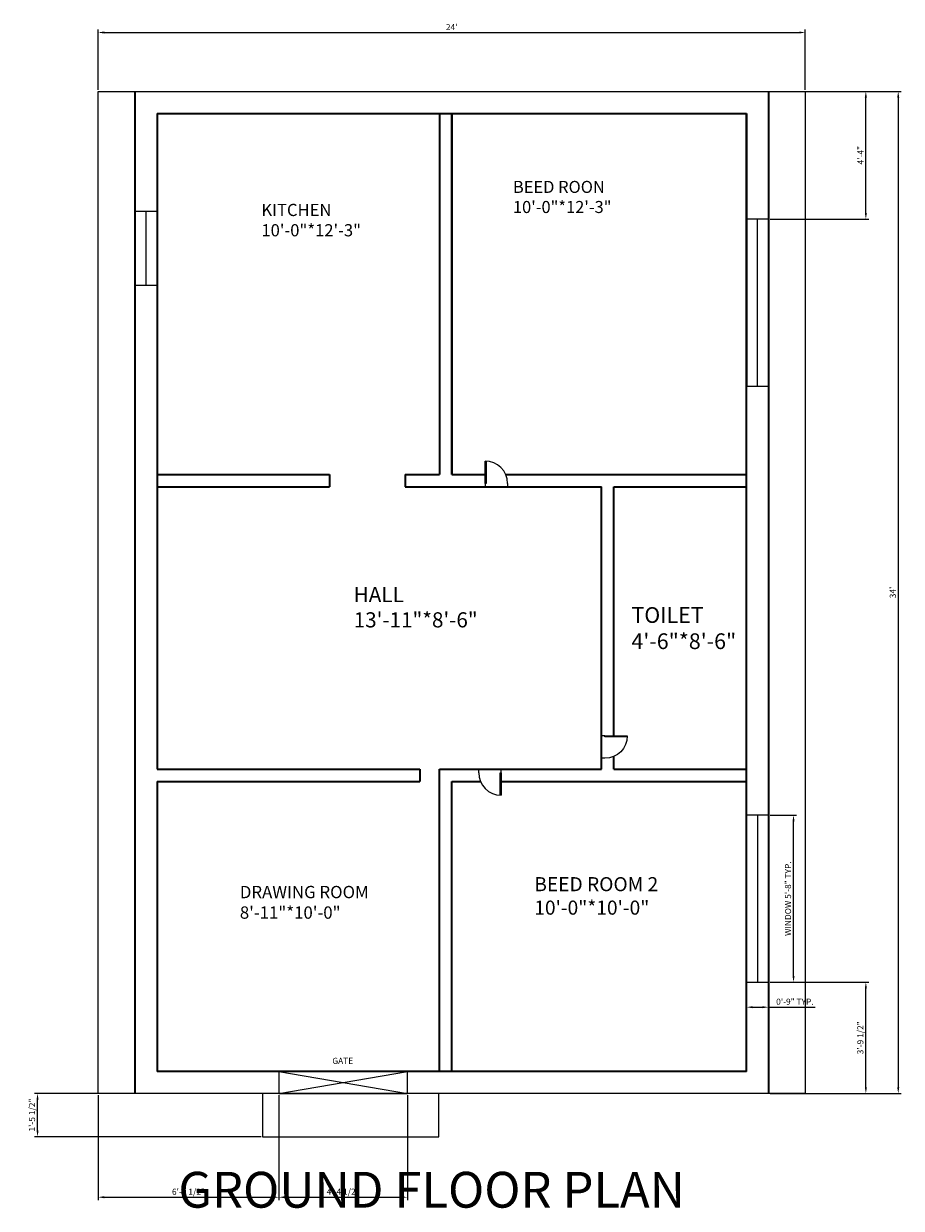
# Model space of a CAD drawing. Units: inches. Extents: x 2432 to 3786, y 1221 to 1905.
# Tile 3 of 4: x 2945 to 3303, y 1397 to 1879. Entities that reach past the tile are written whole.
import ezdxf

# ---------------------------------------------------------------- set-up
doc = ezdxf.new("R2010")
doc.units = ezdxf.units.IN
for name, color, linetype, lineweight, true_color in [('A-ANNO-DIMS', 32, 'Continuous', 18, 0xcd6928), ('A-ANNO-TITL', 40, 'Continuous', 25, 0xf8d731), ('A-AREA-IDEN', 244, 'Continuous', 18, 0x991b1e), ('A-FLOR-STRS', 116, 'Continuous', 18, 0x136734), ('A-GLAZ', 116, 'Continuous', 18, 0x136734), ('A-WALL', 67, 'Continuous', 35, 0x727430), ('C-PROP', 67, 'Continuous', 25, 0x727430), ('L-SITE-GATE', 244, 'Continuous', 18, 0x991b1e)]:
    doc.layers.add(name, color=color, linetype=linetype, lineweight=lineweight, true_color=true_color)
doc.layers.add('A-ANNO-TEXT', color=7, linetype='Continuous', lineweight=18)
doc.layers.add('A-DOOR', color=4, linetype='Continuous', lineweight=18)
doc.styles.get("Standard").update_dxf_attribs({"font": 'arial.ttf'})
doc.dimstyles.new('ISO-25', dxfattribs={"dimtxt": 2.5, "dimasz": 2.5, "dimexe": 1.25, "dimexo": 0.625, "dimtad": 1, "dimdec": 3, "dimlunit": 4, "dimtxsty": 'Standard', "dimcen": 2.5, "dimadec": 0, "dimazin": 0, "dimtfac": 1, "dimtdec": 3, "dimtmove": 0, "dimatfit": 3, "dimfxl": 1, "dimarcsym": 0})

# ---------------------------------------------------------------- blocks, each defined once
blk = doc.blocks.new('*U9')
for p, q in [((0, 0), (0, -6)), ((40, 0), (40, -6))]:
    blk.add_line(p, q)
blk.add_lwpolyline([(0, 0), (0, 40), (1.75, 40), (1.75, 0)], close=True)
blk.add_arc((0, 0), 40, 0, 90)
blk = doc.blocks.new('*U10')
for p, q in [((0, 0), (0, -6)), ((-40, 0), (-40, -6))]:
    blk.add_line(p, q)
blk.add_lwpolyline([(0, 0), (0, 40), (-1.75, 40), (-1.75, 0)], close=True)
blk.add_arc((0, 0), 40, 90, 180)
blk = doc.blocks.new('*D13')
at = {"layer": 'A-ANNO-DIMS', "color": 0, "lineweight": -2, "transparency": 16777216}
for p, q in [((2975.47, 1852.05), (2975.47, 1876.65)), ((3263.47, 1852.05), (3263.47, 1876.65)), ((2977.97, 1875.4), (3260.97, 1875.4))]:
    blk.add_line(p, q, dxfattribs=at)
at = {"layer": 'A-ANNO-DIMS', "color": 0, "lineweight": 5, "transparency": 16777216}
for points in [[(2977.97, 1875.82), (2977.97, 1874.99), (2975.47, 1875.4)], [(3260.97, 1875.82), (3260.97, 1874.99), (3263.47, 1875.4)]]:
    blk.add_solid(points, dxfattribs=at)
at = {"layer": 'Defpoints', "color": 0, "lineweight": 5, "transparency": 16777216}
for p in [(3263.47, 1875.4), (2975.47, 1851.42), (3263.47, 1851.42)]:
    blk.add_point(p, dxfattribs=at)
at = {"layer": 'A-ANNO-DIMS', "color": 0, "transparency": 16777216, "insert": (3119.47, 1877.28), "char_height": 2.5, "attachment_point": 5}
blk.add_mtext("24'", dxfattribs=at)
blk = doc.blocks.new('*D14')
at = {"layer": 'A-ANNO-DIMS', "color": 0, "lineweight": -2, "transparency": 16777216}
for p, q in [((3264.1, 1851.42), (3302.56, 1851.42)), ((3301.31, 1848.92), (3301.31, 1445.92)), ((3264.1, 1443.42), (3302.56, 1443.42))]:
    blk.add_line(p, q, dxfattribs=at)
at = {"layer": 'A-ANNO-DIMS', "color": 0, "lineweight": 5, "transparency": 16777216}
for points in [[(3300.89, 1848.92), (3301.73, 1848.92), (3301.31, 1851.42)], [(3300.89, 1445.92), (3301.73, 1445.92), (3301.31, 1443.42)]]:
    blk.add_solid(points, dxfattribs=at)
at = {"layer": 'Defpoints', "color": 0, "lineweight": 5, "transparency": 16777216}
for p in [(3263.47, 1851.42), (3263.47, 1443.42), (3301.31, 1443.42)]:
    blk.add_point(p, dxfattribs=at)
at = {"layer": 'A-ANNO-DIMS', "color": 0, "transparency": 16777216, "insert": (3299.41, 1647.42), "char_height": 2.5, "attachment_point": 5, "rotation": 90}
blk.add_mtext("34'", dxfattribs=at)
blk = doc.blocks.new('WIN-68')
for p, q in [((9, 67.99), (0, 67.99)), ((0, 67.99), (0, 0)), ((4.5, 67.99), (4.5, 0)), ((9, 0), (9, 67.99)), ((0, 0), (9, 0))]:
    blk.add_line(p, q)
blk = doc.blocks.new('*D27')
at = {"layer": 'A-ANNO-DIMS', "color": 0, "lineweight": -2, "transparency": 16777216}
for p, q in [((3249.1, 1556.76), (3259.92, 1556.76)), ((3258.67, 1491.27), (3258.67, 1554.26)), ((3249.1, 1488.77), (3259.92, 1488.77))]:
    blk.add_line(p, q, dxfattribs=at)
at = {"layer": 'A-ANNO-DIMS', "color": 0, "lineweight": 5, "transparency": 16777216}
for points in [[(3258.25, 1554.26), (3259.09, 1554.26), (3258.67, 1556.76)], [(3258.25, 1491.27), (3259.09, 1491.27), (3258.67, 1488.77)]]:
    blk.add_solid(points, dxfattribs=at)
at = {"layer": 'Defpoints', "color": 0, "lineweight": 5, "transparency": 16777216}
for p in [(3248.47, 1556.76), (3258.67, 1556.76), (3248.47, 1488.77)]:
    blk.add_point(p, dxfattribs=at)
at = {"layer": 'A-ANNO-DIMS', "color": 0, "transparency": 16777216, "insert": (3256.75, 1522.77), "char_height": 2.5, "attachment_point": 5, "rotation": 90}
blk.add_mtext('WINDOW 5\'-8" TYP.', dxfattribs=at)
blk = doc.blocks.new('*D28')
at = {"layer": 'A-ANNO-DIMS', "color": 0, "lineweight": -2, "transparency": 16777216}
for p, q in [((3239.47, 1488.15), (3239.47, 1477.32)), ((3248.47, 1488.15), (3248.47, 1477.32)), ((3241.97, 1478.57), (3245.97, 1478.57)), ((3248.47, 1478.57), (3267.46, 1478.57))]:
    blk.add_line(p, q, dxfattribs=at)
at = {"layer": 'A-ANNO-DIMS', "color": 0, "lineweight": 5, "transparency": 16777216}
for points in [[(3241.97, 1478.99), (3241.97, 1478.16), (3239.47, 1478.57)], [(3245.97, 1478.99), (3245.97, 1478.16), (3248.47, 1478.57)]]:
    blk.add_solid(points, dxfattribs=at)
at = {"layer": 'Defpoints', "color": 0, "lineweight": 5, "transparency": 16777216}
for p in [(3239.47, 1488.77), (3248.47, 1488.77), (3248.47, 1478.57)]:
    blk.add_point(p, dxfattribs=at)
at = {"layer": 'A-ANNO-DIMS', "color": 0, "transparency": 16777216, "insert": (3259.22, 1480.48), "char_height": 2.5, "attachment_point": 5}
blk.add_mtext('0\'-9" TYP.', dxfattribs=at)
blk = doc.blocks.new('*D45')
at = {"layer": 'A-ANNO-DIMS', "color": 0, "lineweight": -2, "transparency": 16777216}
for p, q in [((3041.82, 1443.42), (2949.57, 1443.42)), ((2950.82, 1428.35), (2950.82, 1440.92)), ((3041.82, 1425.85), (2949.57, 1425.85))]:
    blk.add_line(p, q, dxfattribs=at)
at = {"layer": 'A-ANNO-DIMS', "color": 0, "lineweight": 5, "transparency": 16777216}
for points in [[(2950.4, 1440.92), (2951.24, 1440.92), (2950.82, 1443.42)], [(2950.4, 1428.35), (2951.24, 1428.35), (2950.82, 1425.85)]]:
    blk.add_solid(points, dxfattribs=at)
at = {"layer": 'Defpoints', "color": 0, "lineweight": 5, "transparency": 16777216}
for p in [(2950.82, 1443.42), (3042.45, 1443.42), (3042.45, 1425.85)]:
    blk.add_point(p, dxfattribs=at)
at = {"layer": 'A-ANNO-DIMS', "color": 0, "transparency": 16777216, "insert": (2948.9, 1434.64), "char_height": 2.5, "attachment_point": 5, "rotation": 90}
blk.add_mtext('1\'-5 1/2"', dxfattribs=at)
blk = doc.blocks.new('*D46')
at = {"layer": 'A-ANNO-DIMS', "color": 0, "lineweight": -2, "transparency": 16777216}
for p, q in [((3049.07, 1442.8), (3049.07, 1399.95)), ((3101.43, 1442.8), (3101.43, 1399.95)), ((3051.57, 1401.2), (3098.93, 1401.2))]:
    blk.add_line(p, q, dxfattribs=at)
at = {"layer": 'A-ANNO-DIMS', "color": 0, "lineweight": 5, "transparency": 16777216}
for points in [[(3051.57, 1401.62), (3051.57, 1400.79), (3049.07, 1401.2)], [(3098.93, 1401.62), (3098.93, 1400.79), (3101.43, 1401.2)]]:
    blk.add_solid(points, dxfattribs=at)
at = {"layer": 'Defpoints', "color": 0, "lineweight": 5, "transparency": 16777216}
for p in [(3049.07, 1443.42), (3101.43, 1443.42), (3101.43, 1401.2)]:
    blk.add_point(p, dxfattribs=at)
at = {"layer": 'A-ANNO-DIMS', "color": 0, "transparency": 16777216, "insert": (3075.25, 1403.12), "char_height": 2.5, "attachment_point": 5}
blk.add_mtext('4\'-4 1/2"', dxfattribs=at)
blk = doc.blocks.new('*D47')
at = {"layer": 'A-ANNO-DIMS', "color": 0, "lineweight": -2, "transparency": 16777216}
for p, q in [((2975.47, 1442.8), (2975.47, 1399.95)), ((3049.07, 1442.8), (3049.07, 1399.95)), ((2977.97, 1401.2), (3046.57, 1401.2))]:
    blk.add_line(p, q, dxfattribs=at)
at = {"layer": 'A-ANNO-DIMS', "color": 0, "lineweight": 5, "transparency": 16777216}
for points in [[(2977.97, 1401.62), (2977.97, 1400.79), (2975.47, 1401.2)], [(3046.57, 1401.62), (3046.57, 1400.79), (3049.07, 1401.2)]]:
    blk.add_solid(points, dxfattribs=at)
at = {"layer": 'Defpoints', "color": 0, "lineweight": 5, "transparency": 16777216}
for p in [(2975.47, 1443.42), (3049.07, 1443.42), (3049.07, 1401.2)]:
    blk.add_point(p, dxfattribs=at)
at = {"layer": 'A-ANNO-DIMS', "color": 0, "transparency": 16777216, "insert": (3012.27, 1403.12), "char_height": 2.5, "attachment_point": 5}
blk.add_mtext('6\'-1 1/2"', dxfattribs=at)
blk = doc.blocks.new('*D48')
at = {"layer": 'A-ANNO-DIMS', "color": 0, "lineweight": -2, "transparency": 16777216}
for p, q in [((3249.1, 1488.77), (3289.37, 1488.77)), ((3288.12, 1445.92), (3288.12, 1486.27)), ((3249.1, 1443.42), (3289.37, 1443.42))]:
    blk.add_line(p, q, dxfattribs=at)
at = {"layer": 'A-ANNO-DIMS', "color": 0, "lineweight": 5, "transparency": 16777216}
for points in [[(3287.7, 1486.27), (3288.54, 1486.27), (3288.12, 1488.77)], [(3287.7, 1445.92), (3288.54, 1445.92), (3288.12, 1443.42)]]:
    blk.add_solid(points, dxfattribs=at)
at = {"layer": 'Defpoints', "color": 0, "lineweight": 5, "transparency": 16777216}
for p in [(3248.47, 1488.77), (3288.12, 1488.77), (3248.47, 1443.42)]:
    blk.add_point(p, dxfattribs=at)
at = {"layer": 'A-ANNO-DIMS', "color": 0, "transparency": 16777216, "insert": (3286.2, 1466.1), "char_height": 2.5, "attachment_point": 5, "rotation": 90}
blk.add_mtext('3\'-9 1/2"', dxfattribs=at)
blk = doc.blocks.new('*D49')
at = {"layer": 'A-ANNO-DIMS', "color": 0, "lineweight": -2, "transparency": 16777216}
for p, q in [((3249.1, 1851.42), (3289.37, 1851.42)), ((3288.12, 1801.91), (3288.12, 1848.92)), ((3249.1, 1799.41), (3289.37, 1799.41))]:
    blk.add_line(p, q, dxfattribs=at)
at = {"layer": 'A-ANNO-DIMS', "color": 0, "lineweight": 5, "transparency": 16777216}
for points in [[(3287.7, 1848.92), (3288.54, 1848.92), (3288.12, 1851.42)], [(3287.7, 1801.91), (3288.54, 1801.91), (3288.12, 1799.41)]]:
    blk.add_solid(points, dxfattribs=at)
at = {"layer": 'Defpoints', "color": 0, "lineweight": 5, "transparency": 16777216}
for p in [(3248.47, 1851.42), (3288.12, 1851.42), (3248.47, 1799.41)]:
    blk.add_point(p, dxfattribs=at)
at = {"layer": 'A-ANNO-DIMS', "color": 0, "transparency": 16777216, "insert": (3286.25, 1825.42), "char_height": 2.5, "attachment_point": 5, "rotation": 90}
blk.add_mtext('4\'-4"', dxfattribs=at)

msp = doc.modelspace()

# ---------------------------------------------------------------- linework, layer by layer
at = {"layer": 'A-FLOR-STRS'}
for p, q in [((3042.4465, 1443.4238), (3042.4465, 1425.854)), ((3114.229, 1425.854), (3114.229, 1443.4238)), ((3042.4465, 1425.854), (3114.229, 1425.854))]:
    msp.add_line(p, q, dxfattribs=at)
at = {"layer": 'A-GLAZ'}
for p, q in [((2999.4708, 1802.5364), (2990.4708, 1802.5364)), ((2990.4708, 1802.5364), (2990.4708, 1772.5292)), ((2999.4708, 1802.5364), (2994.9708, 1802.5364)), ((2994.9708, 1802.5364), (2994.9708, 1772.5292)), ((2999.4708, 1772.5292), (2999.4708, 1802.5364)), ((3248.4708, 1799.4137), (3243.9708, 1799.4137)), ((2990.4708, 1772.5292), (2999.4708, 1772.5292))]:
    msp.add_line(p, q, dxfattribs=at)
at = {"layer": 'A-WALL'}
for p, q in [((2990.4708, 1851.4238), (2990.4708, 1443.4238)), ((3248.4708, 1851.4238), (3248.4708, 1443.4238)), ((2999.4708, 1842.4238), (2999.4708, 1731.4238)), ((2999.4708, 1842.4238), (2999.4708, 1575.4238)), ((2999.4708, 1842.4238), (3239.4708, 1842.4238)), ((3114.4708, 1842.4238), (3114.4708, 1695.4238)), ((3119.4708, 1842.4238), (3119.4708, 1695.4238)), ((3119.4708, 1695.4238), (3119.4708, 1842.4238)), ((3239.4708, 1842.4238), (3239.4708, 1731.4238)), ((3239.4708, 1452.4238), (3239.4708, 1842.4238)), ((2999.4708, 1695.4238), (3069.6858, 1695.4238)), ((3069.6858, 1695.4238), (3069.6858, 1690.4238)), ((3100.4721, 1695.4238), (3114.4708, 1695.4238)), ((3100.4721, 1695.4238), (3100.4721, 1690.4238)), ((3119.4708, 1695.4238), (3133.0801, 1695.4238)), ((3141.4511, 1695.4238), (3239.4708, 1695.4238)), ((2999.4708, 1690.4238), (3069.6858, 1690.4238)), ((3100.4721, 1690.4238), (3180.4708, 1690.4238)), ((3180.4708, 1575.4238), (3180.4708, 1690.4238)), ((3185.4708, 1690.4238), (3239.4708, 1690.4238)), ((3185.4708, 1589.0039), (3185.4708, 1690.4238)), ((3185.4708, 1575.4238), (3185.4708, 1580.6516)), ((2999.4708, 1575.4238), (3106.4708, 1575.4238)), ((3106.4708, 1575.4238), (3106.4708, 1570.4238)), ((3114.4708, 1570.4238), (3114.4708, 1575.4238)), ((3114.4708, 1575.4238), (3119.4708, 1575.4238)), ((3119.4708, 1575.4238), (3180.4708, 1575.4238)), ((3185.4708, 1575.4238), (3239.4708, 1575.4238)), ((3185.4708, 1575.4238), (3239.4708, 1575.4238)), ((2999.4708, 1570.4238), (3106.4708, 1570.4238)), ((2999.4708, 1570.4238), (2999.4708, 1452.4238)), ((3114.4708, 1452.4238), (3114.4708, 1570.4238)), ((3119.4708, 1452.4238), (3119.4708, 1570.4238)), ((3119.4708, 1570.4238), (3131.2205, 1570.4238)), ((3139.6, 1570.4238), (3239.4708, 1570.4238)), ((3239.4708, 1452.4238), (2999.4708, 1452.4238))]:
    msp.add_line(p, q, dxfattribs=at)
at = {"layer": 'C-PROP'}
for p, q in [((2975.4708, 1851.4238), (3263.4708, 1851.4238)), ((2975.4708, 1443.4238), (2975.4708, 1851.4238)), ((3263.4708, 1851.4238), (3263.4708, 1443.4238)), ((3263.4708, 1443.4238), (2975.4708, 1443.4238))]:
    msp.add_line(p, q, dxfattribs=at)
at = {"layer": 'L-SITE-GATE'}
for p, q in [((3049.0676, 1452.4238), (3049.0676, 1443.4238)), ((3101.433, 1452.4238), (3049.0676, 1452.4238)), ((3049.0676, 1452.4238), (3101.433, 1443.4238)), ((3049.0676, 1443.4238), (3101.433, 1452.4238)), ((3101.433, 1443.4238), (3101.433, 1452.4238)), ((3049.0676, 1443.4238), (3101.433, 1443.4238)), ((3101.433, 1443.4238), (3049.0676, 1443.4238))]:
    msp.add_line(p, q, dxfattribs=at)

# ---------------------------------------------------------------- block references
at = {"layer": 'A-DOOR', "xscale": 0.2277050421196423, "yscale": 0.2277050421196423, "zscale": 0.2277050421196423}
msp.add_blockref('*U9', (3133.0801, 1691.834), dxfattribs=at)
at = {"layer": 'A-DOOR', "yscale": 0.2277050421196423, "zscale": 0.2277050421196423}
for name, p, xscale, rotation in [('*U10', (3181.8378, 1589.0039), -0.2277050421196423, 270), ('*U9', (3139.6, 1573.9936), 0.2277050421196423, 180)]:
    msp.add_blockref(name, p, dxfattribs=dict(at, xscale=xscale, rotation=rotation))
at = {"layer": 'A-GLAZ', "rotation": 180}
msp.add_blockref('WIN-68', (3248.4707, 1799.414), dxfattribs=at)
at = {"layer": 'A-GLAZ'}
msp.add_blockref('WIN-68', (3239.471, 1488.773), dxfattribs=at)

# ---------------------------------------------------------------- texts
at = {"layer": 'A-ANNO-TEXT', "insert": (3070.8754, 1457.9645), "char_height": 2.5, "attachment_point": 1}
msp.add_mtext('{GATE}', dxfattribs=at)
at = {"layer": 'A-ANNO-TITL', "insert": (3008.1453, 1411.5416), "char_height": 14.590252, "attachment_point": 1}
msp.add_mtext_dynamic_manual_height_columns('GROUND FLOOR PLAN', width=282.090868, gutter_width=72.9513, heights=[0], dxfattribs=at)
at = {"layer": 'A-AREA-IDEN', "attachment_point": 1}
for s, width, gutter_width, insert, char_height in [('{BEED ROON\\P10\'-0"*12\'-3"}', 156.743887, 24.5294, (3144.4187, 1814.9884), 4.905877), ('{KITCHEN\\P10\'-0"*12\'-3"}', 93.252996, 24.7943, (3041.9772, 1805.6345), 4.958869), ('{HALL\\P\\pxt7;13\'-11"*8\'-6"}', 155.548591, 30.8627, (3079.5575, 1649.6542), 6.172535), ('{TOILET\\P4\'-6"*8\'-6"}', 58.29074, 31.993, (3192.6732, 1641.4436), 6.398608), ('{BEED ROOM 2\\P10\'-0"*10\'-0"}', 115.157563, 28.6433, (3153.102, 1531.5182), 5.728667), ('{DRAWING ROOM\\P8\'-11"*10\'-0"}', 74.333095, 25.0732, (3033.2048, 1527.96), 5.01464)]:
    msp.add_mtext_dynamic_manual_height_columns(s, width=width, gutter_width=gutter_width, heights=[0], dxfattribs=dict(at, insert=insert, char_height=char_height))

# ---------------------------------------------------------------- dimensions: what is measured, and where the dimension line sits
at = {"layer": 'A-ANNO-DIMS'}
for base, p1, p2, override, picture, middle in [((3263.4708, 1875.4035), (2975.4708, 1851.4238), (3263.4708, 1851.4238), {"dimclrd": 0, "dimclre": 0, "dimclrt": 0}, '*D13', (3119.4708, 1877.2836)), ((3049.0676, 1401.204), (2975.4708, 1443.4238), (3049.0676, 1443.4238), {"dimdec": 1, "dimlfac": 1, "dimrnd": 0, "dimzin": 1, "dimdsep": 46, "dimlunit": 4, "dimfrac": 2}, '*D47', (3012.2692, 1403.1216)), ((3101.433, 1401.204), (3049.0676, 1443.4238), (3101.433, 1443.4238), {"dimdec": 1, "dimlfac": 1, "dimrnd": 0, "dimzin": 1, "dimdsep": 46, "dimlunit": 4, "dimfrac": 2}, '*D46', (3075.2503, 1403.1216))]:
    dim = msp.add_linear_dim(base=base, p1=p1, p2=p2, dimstyle='ISO-25', override=override, dxfattribs=at)
    dim.commit()
    dim.dimension.update_dxf_attribs({"geometry": picture, "text_midpoint": middle})
for base, p1, p2, override, picture, middle in [((3288.1208, 1851.4238), (3248.4708, 1799.4137), (3248.4708, 1851.4238), {"dimdec": 1, "dimlfac": 1, "dimrnd": 0, "dimzin": 1, "dimdsep": 46, "dimlunit": 4, "dimfrac": 2}, '*D49', (3286.2458, 1825.4187)), ((3301.311, 1443.4238), (3263.4708, 1851.4238), (3263.4708, 1443.4238), {"dimclrd": 0, "dimclre": 0, "dimclrt": 0}, '*D14', (3299.4087, 1647.4238)), ((3288.1208, 1488.7733), (3248.4708, 1443.4238), (3248.4708, 1488.7733), {"dimdec": 1, "dimlfac": 1, "dimrnd": 0, "dimzin": 1, "dimdsep": 46, "dimlunit": 4, "dimfrac": 2}, '*D48', (3286.2023, 1466.0985)), ((2950.8208, 1443.4238), (3042.4465, 1425.854), (3042.4465, 1443.4238), {"dimdec": 1, "dimlfac": 1, "dimrnd": 0, "dimzin": 1, "dimdsep": 46, "dimlunit": 4, "dimfrac": 2}, '*D45', (2948.9032, 1434.6389))]:
    dim = msp.add_linear_dim(base=base, p1=p1, p2=p2, angle=90, dimstyle='ISO-25', override=override, dxfattribs=at)
    dim.commit()
    dim.dimension.update_dxf_attribs({"geometry": picture, "text_midpoint": middle})
dim = msp.add_linear_dim(base=(3258.6693, 1556.7633), p1=(3248.4708, 1488.7733), p2=(3248.4708, 1556.7633), angle=90, text='WINDOW <> TYP.', dimstyle='ISO-25', override={"dimdec": 1, "dimlfac": 1, "dimrnd": 0, "dimzin": 1, "dimdsep": 46, "dimlunit": 4, "dimfrac": 2}, dxfattribs=at)
dim.commit()
dim.dimension.update_dxf_attribs({"geometry": '*D27', "text_midpoint": (3256.7508, 1522.7683)})
dim = msp.add_linear_dim(base=(3248.4708, 1478.5748), p1=(3239.4708, 1488.7733), p2=(3248.4708, 1488.7733), text='<> TYP.', dimstyle='ISO-25', override={"dimdec": 1, "dimlfac": 1, "dimrnd": 0, "dimzin": 1, "dimdsep": 46, "dimlunit": 4, "dimfrac": 2}, dxfattribs=at)
dim.commit()
dim.dimension.update_dxf_attribs({"geometry": '*D28', "text_midpoint": (3259.2152, 1480.4763)})

doc.saveas('drawing.dxf')
